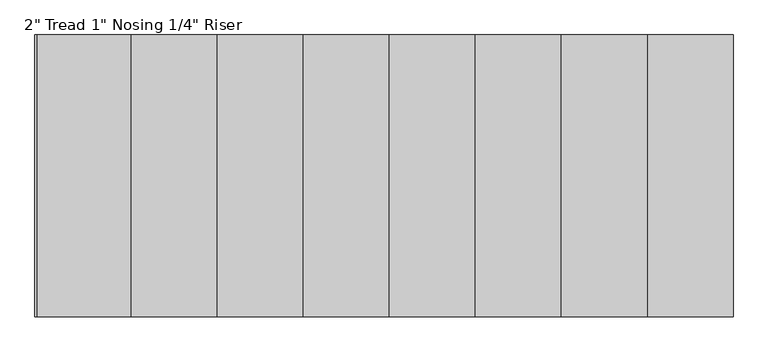
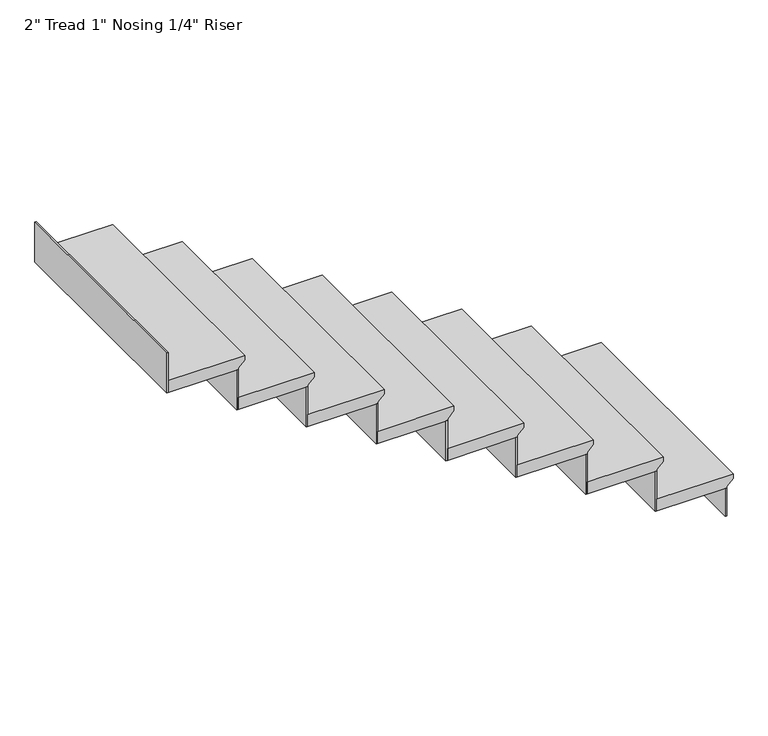
"""IFC4 building model written with IfcOpenShell, lengths in millimetres: stair flight geometry."""

from ifc_helpers import new_model, si_unit, frame, origin, origin_with_axes, place, context, project, spatial, polyline, outline, extrude, source, transform, mapped, element, save


def stair_flight_e425de01(model_context):
    return source(origin(), model_context, "Body", "SweptSolid", [
        extrude(outline(polyline([(169.3333333, -9406.5505662), (169.3333333, -9711.3505662), (118.5333333, -9711.3505662), (118.5333333, -9431.9505662), (124.8833333, -9431.9505662), (150.2833333, -9406.5505662), (169.3333333, -9406.5505662)])), frame((0.0, 576.9742707, 0.0), z_axis=(0.0, 1.0, 0.0), x_axis=(0.0, 0.0, 1.0)), (0.0, 0.0, 1.0), 914.4),
        extrude(outline(polyline([(-9438.3005662, 1491.3742707), (-9431.9505662, 1491.3742707), (-9431.9505662, 576.9742707), (-9438.3005662, 576.9742707), (-9438.3005662, 1491.3742707)])), origin_with_axes(), (0.0, 0.0, 1.0), 118.5333333),
        extrude(outline(polyline([(-9717.7005662, 1491.3742707), (-9711.3505662, 1491.3742707), (-9711.3505662, 576.9742707), (-9717.7005662, 576.9742707), (-9717.7005662, 1491.3742707)])), frame((0.0, 0.0, 118.5333333), z_axis=(0.0, 0.0, 1.0), x_axis=(1.0, 0.0, 0.0)), (0.0, 0.0, 1.0), 169.3333333),
        extrude(outline(polyline([(338.6666667, -9685.9505662), (338.6666667, -9990.7505662), (287.8666667, -9990.7505662), (287.8666667, -9711.3505662), (294.2166667, -9711.3505662), (319.6166667, -9685.9505662), (338.6666667, -9685.9505662)])), frame((0.0, 576.9742707, 0.0), z_axis=(0.0, 1.0, 0.0), x_axis=(0.0, 0.0, 1.0)), (0.0, 0.0, 1.0), 914.4),
        extrude(outline(polyline([(-9997.1005662, 1491.3742707), (-9990.7505662, 1491.3742707), (-9990.7505662, 576.9742707), (-9997.1005662, 576.9742707), (-9997.1005662, 1491.3742707)])), frame((0.0, 0.0, 287.8666667), z_axis=(0.0, 0.0, 1.0), x_axis=(1.0, 0.0, 0.0)), (0.0, 0.0, 1.0), 169.3333333),
        extrude(outline(polyline([(508.0, -9965.3505662), (508.0, -10270.1505662), (457.2, -10270.1505662), (457.2, -9990.7505662), (463.55, -9990.7505662), (488.95, -9965.3505662), (508.0, -9965.3505662)])), frame((0.0, 576.9742707, 0.0), z_axis=(0.0, 1.0, 0.0), x_axis=(0.0, 0.0, 1.0)), (0.0, 0.0, 1.0), 914.4),
        extrude(outline(polyline([(-10276.5005662, 1491.3742707), (-10270.1505662, 1491.3742707), (-10270.1505662, 576.9742707), (-10276.5005662, 576.9742707), (-10276.5005662, 1491.3742707)])), frame((0.0, 0.0, 457.2), z_axis=(0.0, 0.0, 1.0), x_axis=(1.0, 0.0, 0.0)), (0.0, 0.0, 1.0), 169.3333333),
        extrude(outline(polyline([(677.3333333, -10244.7505662), (677.3333333, -10549.5505662), (626.5333333, -10549.5505662), (626.5333333, -10270.1505662), (632.8833333, -10270.1505662), (658.2833333, -10244.7505662), (677.3333333, -10244.7505662)])), frame((0.0, 576.9742707, 0.0), z_axis=(0.0, 1.0, 0.0), x_axis=(0.0, 0.0, 1.0)), (0.0, 0.0, 1.0), 914.4),
        extrude(outline(polyline([(-10555.9005662, 1491.3742707), (-10549.5505662, 1491.3742707), (-10549.5505662, 576.9742707), (-10555.9005662, 576.9742707), (-10555.9005662, 1491.3742707)])), frame((0.0, 0.0, 626.5333333), z_axis=(0.0, 0.0, 1.0), x_axis=(1.0, 0.0, 0.0)), (0.0, 0.0, 1.0), 169.3333333),
        extrude(outline(polyline([(846.6666667, -10524.1505662), (846.6666667, -10828.9505662), (795.8666667, -10828.9505662), (795.8666667, -10549.5505662), (802.2166667, -10549.5505662), (827.6166667, -10524.1505662), (846.6666667, -10524.1505662)])), frame((0.0, 576.9742707, 0.0), z_axis=(0.0, 1.0, 0.0), x_axis=(0.0, 0.0, 1.0)), (0.0, 0.0, 1.0), 914.4),
        extrude(outline(polyline([(-10835.3005662, 1491.3742707), (-10828.9505662, 1491.3742707), (-10828.9505662, 576.9742707), (-10835.3005662, 576.9742707), (-10835.3005662, 1491.3742707)])), frame((0.0, 0.0, 795.8666667), z_axis=(0.0, 0.0, 1.0), x_axis=(1.0, 0.0, 0.0)), (0.0, 0.0, 1.0), 169.3333333),
        extrude(outline(polyline([(1016.0, -10803.5505662), (1016.0, -11108.3505662), (965.2, -11108.3505662), (965.2, -10828.9505662), (971.55, -10828.9505662), (996.95, -10803.5505662), (1016.0, -10803.5505662)])), frame((0.0, 576.9742707, 0.0), z_axis=(0.0, 1.0, 0.0), x_axis=(0.0, 0.0, 1.0)), (0.0, 0.0, 1.0), 914.4),
        extrude(outline(polyline([(-11114.7005662, 1491.3742707), (-11108.3505662, 1491.3742707), (-11108.3505662, 576.9742707), (-11114.7005662, 576.9742707), (-11114.7005662, 1491.3742707)])), frame((0.0, 0.0, 965.2), z_axis=(0.0, 0.0, 1.0), x_axis=(1.0, 0.0, 0.0)), (0.0, 0.0, 1.0), 169.3333333),
        extrude(outline(polyline([(1185.3333333, -11082.9505662), (1185.3333333, -11387.7505662), (1134.5333333, -11387.7505662), (1134.5333333, -11108.3505662), (1140.8833333, -11108.3505662), (1166.2833333, -11082.9505662), (1185.3333333, -11082.9505662)])), frame((0.0, 576.9742707, 0.0), z_axis=(0.0, 1.0, 0.0), x_axis=(0.0, 0.0, 1.0)), (0.0, 0.0, 1.0), 914.4),
        extrude(outline(polyline([(-11394.1005662, 1491.3742707), (-11387.7505662, 1491.3742707), (-11387.7505662, 576.9742707), (-11394.1005662, 576.9742707), (-11394.1005662, 1491.3742707)])), frame((0.0, 0.0, 1134.5333333), z_axis=(0.0, 0.0, 1.0), x_axis=(1.0, 0.0, 0.0)), (0.0, 0.0, 1.0), 169.3333333),
        extrude(outline(polyline([(-11673.5005662, 1491.3742707), (-11667.1505662, 1491.3742707), (-11667.1505662, 576.9742707), (-11673.5005662, 576.9742707), (-11673.5005662, 1491.3742707)])), frame((0.0, 0.0, 1303.8666667), z_axis=(0.0, 0.0, 1.0), x_axis=(1.0, 0.0, 0.0)), (0.0, 0.0, 1.0), 169.3333333),
        extrude(outline(polyline([(1354.6666667, -11362.3505662), (1354.6666667, -11667.1505662), (1303.8666667, -11667.1505662), (1303.8666667, -11387.7505662), (1310.2166667, -11387.7505662), (1335.6166667, -11362.3505662), (1354.6666667, -11362.3505662)])), frame((0.0, 576.9742707, 0.0), z_axis=(0.0, 1.0, 0.0), x_axis=(0.0, 0.0, 1.0)), (0.0, 0.0, 1.0), 914.4),
    ])


if __name__ == "__main__":
    model = new_model("IFC4")
    model_context = context("Model", 3, world=origin())
    ifc_project = project(units=[si_unit("LENGTHUNIT", "METRE", prefix="MILLI")], contexts=[model_context])
    site = spatial("IfcSite", under=ifc_project)
    building = spatial("IfcBuilding", under=site)
    placement = place(None, origin())
    stair_flight_shape = stair_flight_e425de01(model_context)
    element("IfcStairFlight", 1, ObjectType="2\" Tread 1\" Nosing 1/4\" Riser", at=placement, inside=building, context=model_context, shape_type="MappedRepresentation", body=[
        mapped(stair_flight_shape, transform((0.0, 0.0, 0.0), x_axis=(1.0, 0.0, 0.0), y_axis=(0.0, 1.0, 0.0), z_axis=(0.0, 0.0, 1.0))),
    ])
    save(model, "model.ifc")
